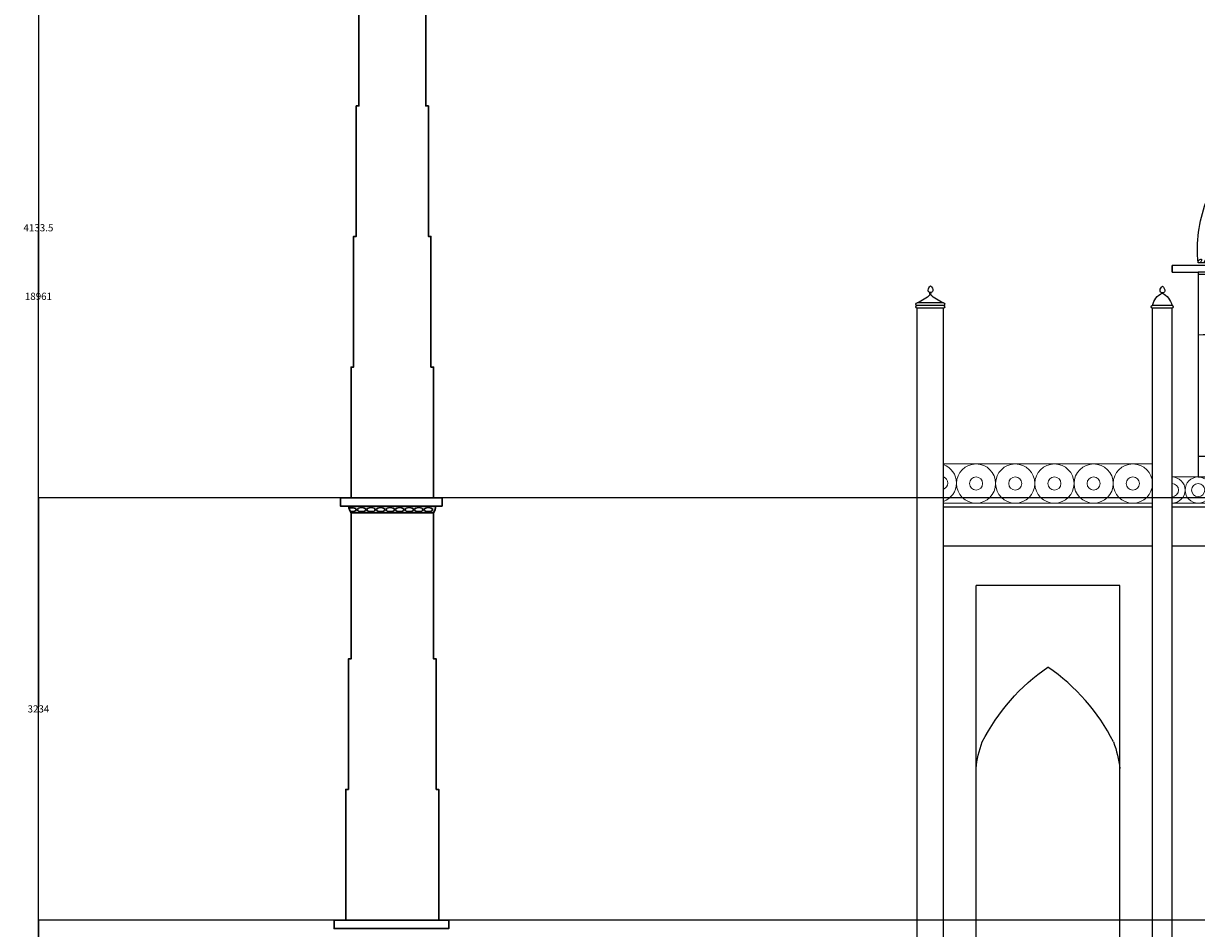
# Model space of a CAD drawing. Units: millimetres. Extents: x 8570 to 49085, y 3782 to 24863.
# Tile 2 of 15: x 8570 to 17549, y 10542 to 17471. Entities that reach past the tile are written whole.
import ezdxf

# ---------------------------------------------------------------- set-up
doc = ezdxf.new("R2010")
doc.units = ezdxf.units.MM
doc.header["$MEASUREMENT"] = 0
doc.header["$PDMODE"] = 3
for name, color, linetype, lineweight in [('A-ANNO-DIMS', 2, 'Continuous', 18), ('A-ELEV', 7, 'Continuous', 25), ('A-ELEV-ARCH', 7, 'Continuous', 25), ('A-ELEV-MNRT', 7, 'Continuous', 30), ('A-ELEV-ORNM', 7, 'Continuous', 13), ('A-ELEV-PIER', 7, 'Continuous', 25), ('A-ROOF-CHAT', 7, 'Continuous', 25)]:
    doc.layers.add(name, color=color, linetype=linetype, lineweight=lineweight)
doc.styles.get("Standard").update_dxf_attribs({"font": 'arial.ttf'})
doc.dimstyles.get("Standard").update_dxf_attribs({"dimtxt": 55, "dimasz": 0.18, "dimexe": 0.18, "dimexo": 0.0625, "dimgap": 0.09, "dimtad": 0, "dimtih": 1, "dimtoh": 1, "dimdec": 0, "dimzin": 0, "dimdsep": 46, "dimtxsty": 'Standard', "dimcen": 0.09, "dimadec": 0, "dimazin": 0, "dimtfac": 1, "dimtdec": 0, "dimtofl": 0, "dimtmove": 0, "dimatfit": 3, "dimfxl": 1, "dimtolj": 1, "dimtzin": 0, "dimarcsym": 0})

# ---------------------------------------------------------------- blocks, each defined once
blk = doc.blocks.new('MINARET-ELEV')
h = blk.add_hatch(color=256)
h.dxf.hatch_style = 1
edge = h.paths.add_edge_path()
edge.add_arc((788.1, 7879), 96, 347.52389, 357.31225, ccw=False)
edge.add_ellipse((859.2, 7847.7), major_axis=(31.8, 0), ratio=0.472441, start_angle=385.01443, end_angle=315.51296)
edge.add_arc((788.1, 7879), 96, 325.26025, 332.17741, ccw=False)
edge.add_line((867, 7824.3), (235, 7824.3))
edge.add_arc((313.9, 7879), 96, 182.68775, 214.73975, ccw=False)
edge.add_line((218, 7874.5), (884, 7874.5))
edge = h.paths.add_edge_path(flags=16)
edge.add_ellipse((494.2, 7847.7), major_axis=(31.8, 0), ratio=0.472441, start_angle=0, end_angle=360, ccw=False)
edge = h.paths.add_edge_path(flags=16)
edge.add_ellipse((567.2, 7847.7), major_axis=(31.8, 0), ratio=0.472441, start_angle=0, end_angle=360, ccw=False)
edge = h.paths.add_edge_path(flags=16)
edge.add_ellipse((421.2, 7847.7), major_axis=(31.8, 0), ratio=0.472441, start_angle=0, end_angle=360, ccw=False)
edge = h.paths.add_edge_path(flags=16)
edge.add_ellipse((640.2, 7847.7), major_axis=(31.8, 0), ratio=0.472441, start_angle=0, end_angle=360, ccw=False)
edge = h.paths.add_edge_path(flags=16)
edge.add_ellipse((348.2, 7847.7), major_axis=(31.8, 0), ratio=0.472441, start_angle=0, end_angle=360, ccw=False)
edge = h.paths.add_edge_path(flags=16)
edge.add_ellipse((713.2, 7847.7), major_axis=(31.8, 0), ratio=0.472441, start_angle=0, end_angle=360, ccw=False)
edge = h.paths.add_edge_path(flags=16)
edge.add_ellipse((275.2, 7847.7), major_axis=(31.8, 0), ratio=0.472441, start_angle=0, end_angle=360, ccw=False)
edge = h.paths.add_edge_path(flags=16)
edge.add_ellipse((786.2, 7847.7), major_axis=(31.8, 0), ratio=0.472441, start_angle=0, end_angle=360, ccw=False)
blk.add_line((867, 7824.3), (235, 7824.3))
blk.add_line((867, 7824.3), (235, 7824.3))
for points in [[(235, 7939), (235, 8939), (255, 8939), (255, 9939), (275, 9939), (275, 10939), (295, 10939), (295, 11939)], [(867, 7939), (867, 8939), (847, 8939), (847, 9939), (827, 9939), (827, 10939), (807, 10939), (807, 11939)], [(195, 4705), (195, 5705), (215, 5705), (215, 6705), (235, 6705), (235, 7824.3)], [(907, 4705), (907, 5705), (887, 5705), (887, 6705), (867, 6705), (867, 7824.3)]]:
    blk.add_lwpolyline(points)
for points in [[(948, 7939), (170.5, 7939), (170.5, 7874.5), (948, 7874.5)], [(997, 4705), (119.5, 4705), (119.5, 4640.5), (997, 4640.5)]]:
    blk.add_lwpolyline(points, close=True)
for centre, start, end in [((313.9, 7879), 182.68775, 214.73975), ((788.1, 7879), 325.26025, 357.31225)]:
    blk.add_arc(centre, 96, start, end)
at = {"extrusion": (0, 0, -1)}
for centre, start_param, end_param in [((275.2, 7847.7), -6.283185, 0), ((348.2, 7847.7), -6.283185, 0), ((421.2, 7847.7), -6.283185, 0), ((494.2, 7847.7), -6.283185, 0), ((567.2, 7847.7), -6.283185, 0), ((640.2, 7847.7), -6.283185, 0), ((713.2, 7847.7), -6.283185, 0), ((786.2, 7847.7), -6.283185, 0), ((859.2, 7847.7), -5.160703, -0.779193)]:
    blk.add_ellipse(centre, major_axis=(31.8, 0), ratio=0.472441, start_param=start_param, end_param=end_param, dxfattribs=at)
blk = doc.blocks.new('PAVILION-EDGE-PINNACLE')
for p, q in [((10, 8089.5), (160, 8089.5)), ((10, 0), (10, 8069.5)), ((10, 8069.5), (160, 8069.5)), ((160, 0), (160, 8069.5)), ((160, 0), (160, 6876.5)), ((10, 0), (10, 6246.5))]:
    blk.add_line(p, q)
blk.add_lwpolyline([(101.6, 8204.8, 0.216309), (82.9, 8236.3, 0.244698), (64, 8200, 0.244698)], format="xyb")
for centre, radius, start, end in [((153, 8055.1), 147, 117.52778, 166.47476), ((82.6, 8204.4), 19, 193.30654, 1.38797), ((17, 8055.1), 147, 13.52524, 62.47222), ((10, 8079.5), 10, 90, 270), ((160, 8079.5), 10, 270, 90)]:
    blk.add_arc(centre, radius, start, end)
blk = doc.blocks.new('WING-END-PINNACLE')
for p, q in [((10, 8109.5), (210, 8109.5)), ((10, 8089.5), (210, 8089.5)), ((10, 0), (10, 8069.5)), ((10, 8069.5), (210, 8069.5)), ((210, 0), (210, 8069.5))]:
    blk.add_line(p, q)
blk.add_lwpolyline([(127.1, 8207.4, 0.216309), (108.4, 8238.9, 0.244698), (89.5, 8202.5, 0.244698)], format="xyb")
blk.add_circle((110.5, 8181), 7.02)
for centre, radius, start, end in [((-119.7, 8420.4), 336.9, 292.6494, 312.99463), ((108.1, 8206.9), 19, 193.30654, 1.38797), ((340.2, 8421.1), 337.7, 227.0303, 247.32566), ((10, 8099.5), 10, 90, 270), ((10, 8079.5), 10, 90, 270), ((210, 8099.5), 10, 270, 90), ((210, 8079.5), 10, 270, 90)]:
    blk.add_arc(centre, radius, start, end)
blk = doc.blocks.new('ARCADE-RING-FRIEZE')
for p, q in [((0, 200), (2300, 200)), ((2300, 200), (2100, 200)), ((0, 0), (2300, 0))]:
    blk.add_line(p, q)
for centre, radius in [((100, 100), 100), ((300, 100), 100), ((500, 100), 100), ((700, 100), 100), ((900, 100), 100), ((1100, 100), 100), ((1300, 100), 100), ((1500, 100), 100), ((1700, 100), 100), ((1900, 100), 100), ((2100, 100), 100), ((100, 100), 50), ((300, 100), 50), ((500, 100), 50), ((700, 100), 50), ((900, 100), 50), ((1100, 100), 50), ((1300, 100), 50), ((1500, 100), 50), ((1700, 100), 50), ((1900, 100), 50), ((2100, 100), 50)]:
    blk.add_circle(centre, radius)
for radius in [100, 50]:
    blk.add_arc((2300, 100), radius, 90, 270)
blk = doc.blocks.new('WING-RING-FRIEZE')
for p, q in [((0, 300), (1600, 300)), ((0, 0), (1600, 0))]:
    blk.add_line(p, q)
for centre, radius in [((150, 150), 150), ((450, 150), 150), ((750, 150), 150), ((1050, 150), 150), ((1349.9, 150), 150), ((150, 150), 50), ((450, 150), 50), ((750, 150), 50), ((1050, 150), 50), ((1349.9, 150), 50)]:
    blk.add_circle(centre, radius)
for centre, radius in [((1649.9, 153.7), 150), ((1616.6, 153.7), 50)]:
    blk.add_arc(centre, radius, 109.41717, 250.58283)
blk = doc.blocks.new('CHHATRI-ELEV')
for p, q in [((1107.1, 3111.9), (1194.6, 3111.9)), ((819.3, 2507.3), (1150, 2958.1)), ((967.4, 2449.5), (1150, 2958.1)), ((1480.7, 2507.3), (1150, 2958.1)), ((1339.8, 2454.2), (1150, 2958.1)), ((200, 1639.5), (2100, 1639.5)), ((2300, 1569.5), (2300, 1619.5)), ((200, 1549.5), (2100, 1549.5)), ((610, 0), (610, 754)), ((800, 0), (800, 754)), ((1500, 0), (1500, 744.5)), ((1692, 0), (1692, 744.5)), ((610, 158.5), (200, 158.5)), ((800, 158.5), (1500, 158.5)), ((2100, 158.5), (1692, 158.5))]:
    blk.add_line(p, q)
for points in [[(1199.3, 3183.7, 0.216309), (1151.6, 3264, 0.244698), (1103.6, 3171.4, 0.244698)], [(1198.5, 3007.8, 0.216309), (1150.8, 3088.1, 0.244698), (1102.8, 2995.4, 0.244698)], [(259.6, 2102.5, -0.128405), (908.9, 2832.4, 0.03556), (1150, 2958.1)], [(2040.4, 2102.5, 0.128405), (1391.1, 2832.4, -0.03556), (1150, 2958.1)]]:
    blk.add_lwpolyline(points, format="xyb")
for points in [[(200, 1569.5), (0, 1569.5), (0, 1619.5), (2300, 1619.5), (2300, 1569.5), (2100, 1569.5)], [(2100, 0), (200, 0), (200, 1569.5), (2100, 1569.5), (2100, 0)]]:
    blk.add_lwpolyline(points)
for points in [[(225.8, 1639.5, 0.520567), (200.9, 1667.5, 0.520567)], [(273.9, 1639.5, 0.520567), (249, 1667.5, 0.520567)], [(321.9, 1639.5, 0.520567), (297.1, 1667.5, 0.520567)], [(370, 1639.5, 0.520567), (345.1, 1667.5, 0.520567)], [(418, 1639.5, 0.520567), (393.2, 1667.5, 0.520567)], [(466.1, 1639.5, 0.520567), (441.2, 1667.5, 0.520567)], [(514.2, 1639.5, 0.520567), (489.3, 1667.5, 0.520567)], [(562.2, 1639.5, 0.520567), (537.3, 1667.5, 0.520567)], [(610.3, 1639.5, 0.520567), (585.4, 1667.5, 0.520567)], [(658.3, 1639.5, 0.520567), (633.4, 1667.5, 0.520567)], [(706.4, 1639.5, 0.520567), (681.5, 1667.5, 0.520567)], [(754.4, 1639.5, 0.520567), (729.6, 1667.5, 0.520567)], [(802.5, 1639.5, 0.520567), (777.6, 1667.5, 0.520567)], [(850.5, 1639.5, 0.520567), (825.7, 1667.5, 0.520567)], [(898.6, 1639.5, 0.520567), (873.7, 1667.5, 0.520567)], [(946.7, 1639.5, 0.520567), (921.8, 1667.5, 0.520567)], [(994.7, 1639.5, 0.520567), (969.8, 1667.5, 0.520567)], [(1042.8, 1639.5, 0.520567), (1017.9, 1667.5, 0.520567)], [(1090.8, 1639.5, 0.520567), (1065.9, 1667.5, 0.520567)], [(1138.9, 1639.5, 0.520567), (1114, 1667.5, 0.520567)], [(1186.9, 1639.5, 0.520567), (1162.1, 1667.5, 0.520567)], [(1235, 1639.5, 0.520567), (1210.1, 1667.5, 0.520567)], [(1283, 1639.5, 0.520567), (1258.2, 1667.5, 0.520567)], [(1331.1, 1639.5, 0.520567), (1306.2, 1667.5, 0.520567)], [(1379.2, 1639.5, 0.520567), (1354.3, 1667.5, 0.520567)], [(1427.2, 1639.5, 0.520567), (1402.3, 1667.5, 0.520567)], [(1475.3, 1639.5, 0.520567), (1450.4, 1667.5, 0.520567)], [(1523.3, 1639.5, 0.520567), (1498.4, 1667.5, 0.520567)], [(1571.4, 1639.5, 0.520567), (1546.5, 1667.5, 0.520567)], [(1619.4, 1639.5, 0.520567), (1594.6, 1667.5, 0.520567)], [(1667.5, 1639.5, 0.520567), (1642.6, 1667.5, 0.520567)], [(1715.6, 1639.5, 0.520567), (1690.7, 1667.5, 0.520567)], [(1763.6, 1639.5, 0.520567), (1738.7, 1667.5, 0.520567)], [(1811.7, 1639.5, 0.520567), (1786.8, 1667.5, 0.520567)], [(1859.7, 1639.5, 0.520567), (1834.8, 1667.5, 0.520567)], [(1907.8, 1639.5, 0.520567), (1882.9, 1667.5, 0.520567)], [(1955.8, 1639.5, 0.520567), (1931, 1667.5, 0.520567)], [(2003.9, 1639.5, 0.520567), (1979, 1667.5, 0.520567)], [(2051.9, 1639.5, 0.520567), (2027.1, 1667.5, 0.520567)], [(2100, 1639.5, 0.520567), (2075.1, 1667.5, 0.520567)]]:
    blk.add_lwpolyline(points, format="xyb", close=True)
blk.add_circle((1150.8, 3100), 11.9)
for centre, radius, start, end in [((1150.8, 3182.5), 48.5, 193.30654, 1.38797), ((1150.8, 3079.7), 54.3, 36.37477, 143.62523), ((1150, 3006.6), 48.5, 193.30654, 1.38797), ((1145, 3123.8), 717.3, 225.15569, 315.39684), ((1145, 3123.8), 697.3, 225.15569, 315.39684), ((1217.2, 1743.8), 1022.5, 159.46554, 185.85431), ((1082.8, 1743.8), 1022.5, 354.14569, 20.53446), ((260.1, 742.6), 350.1, 358.13323, 99.88317), ((1149.9, 742.6), 350.1, 359.68831, 181.86677), ((2042.1, 742.6), 350.1, 80.47888, 180.31169)]:
    blk.add_arc(centre, radius, start, end)
blk = doc.blocks.new('WING-TALL-ARCH')
for p, q in [((0, 5946.5), (1100, 5946.5)), ((0, 0), (0, 5946.5)), ((1100, 0), (1100, 5946.5)), ((0, 3123.2), (1100, 3123.2))]:
    blk.add_line(p, q)
for points in [[(47.9, 4748, -0.124525), (550, 5321.3, -0.124525)], [(1052.1, 4748, 0.124525), (550, 5321.3, 0.124525)]]:
    blk.add_lwpolyline(points, format="xyb")
for centre, start, end in [((817.4, 4459.8), 159.46554, 174.14569), ((282.6, 4459.8), 5.85431, 20.53446)]:
    blk.add_arc(centre, 821.7, start, end)
blk = doc.blocks.new('*D44')
at = {"layer": 'A-ANNO-DIMS', "color": 0, "lineweight": -2, "transparency": 16777216}
for p, q in [((22399.7, 24863), (8684.3, 24863)), ((8684.5, 24862.8), (8684.5, 15410.4)), ((8684.5, 5901.7), (8684.5, 15354.1)), ((10843.9, 5901.5), (8684.3, 5901.5))]:
    blk.add_line(p, q, dxfattribs=at)
at = {"layer": 'A-ANNO-DIMS', "color": 0, "transparency": 16777216}
for points in [[(8684.5, 24862.8), (8684.5, 24862.8), (8684.5, 24863)], [(8684.5, 5901.7), (8684.5, 5901.7), (8684.5, 5901.5)]]:
    blk.add_solid(points, dxfattribs=at)
at = {"layer": 'Defpoints', "color": 0, "transparency": 16777216}
for p in [(8684.5, 24863), (22399.8, 24863), (10844, 5901.5)]:
    blk.add_point(p, dxfattribs=at)
at = {"layer": 'A-ANNO-DIMS', "color": 0, "transparency": 16777216, "insert": (8684.5, 15382.2), "char_height": 55, "attachment_point": 5}
blk.add_mtext('\\A1;18961', dxfattribs=at)
blk = doc.blocks.new('*D59')
at = {"layer": 'A-ANNO-DIMS', "color": 0, "lineweight": -2, "transparency": 16777216}
for p, q in [((32990.4, 10606.5), (8684.3, 10606.5)), ((8684.5, 10606.3), (8684.5, 8942.7)), ((8684.5, 7222.7), (8684.5, 8886.3)), ((32870.9, 7222.5), (8684.3, 7222.5))]:
    blk.add_line(p, q, dxfattribs=at)
at = {"layer": 'A-ANNO-DIMS', "color": 0, "transparency": 16777216}
for points in [[(8684.5, 10606.3), (8684.5, 10606.3), (8684.5, 10606.5)], [(8684.5, 7222.7), (8684.5, 7222.7), (8684.5, 7222.5)]]:
    blk.add_solid(points, dxfattribs=at)
at = {"layer": 'Defpoints', "color": 0, "transparency": 16777216}
for p in [(8684.5, 10606.5), (32990.5, 10606.5), (32871, 7222.5)]:
    blk.add_point(p, dxfattribs=at)
at = {"layer": 'A-ANNO-DIMS', "color": 0, "transparency": 16777216, "insert": (8684.5, 8914.5), "char_height": 55, "attachment_point": 5}
blk.add_mtext('\\A1;3384', dxfattribs=at)
blk = doc.blocks.new('*D60')
at = {"layer": 'A-ANNO-DIMS', "color": 0, "lineweight": -2, "transparency": 16777216}
for p, q in [((33041.4, 13840.5), (8684.3, 13840.5)), ((8684.5, 13840.3), (8684.5, 12251.7)), ((8684.5, 10606.7), (8684.5, 12195.3)), ((32990.4, 10606.5), (8684.3, 10606.5))]:
    blk.add_line(p, q, dxfattribs=at)
at = {"layer": 'A-ANNO-DIMS', "color": 0, "transparency": 16777216}
for points in [[(8684.5, 13840.3), (8684.5, 13840.3), (8684.5, 13840.5)], [(8684.5, 10606.7), (8684.5, 10606.7), (8684.5, 10606.5)]]:
    blk.add_solid(points, dxfattribs=at)
at = {"layer": 'Defpoints', "color": 0, "transparency": 16777216}
for p in [(8684.5, 13840.5), (33041.5, 13840.5), (32990.5, 10606.5)]:
    blk.add_point(p, dxfattribs=at)
at = {"layer": 'A-ANNO-DIMS', "color": 0, "transparency": 16777216, "insert": (8684.5, 12223.5), "char_height": 55, "attachment_point": 5}
blk.add_mtext('\\A1;3234', dxfattribs=at)
blk = doc.blocks.new('*D61')
at = {"layer": 'A-ANNO-DIMS', "color": 0, "lineweight": -2, "transparency": 16777216}
for p, q in [((33091.4, 17974), (8684.3, 17974)), ((8684.5, 17973.8), (8684.5, 15935.4)), ((8684.5, 13840.7), (8684.5, 15879.1)), ((33041.4, 13840.5), (8684.3, 13840.5))]:
    blk.add_line(p, q, dxfattribs=at)
at = {"layer": 'A-ANNO-DIMS', "color": 0, "transparency": 16777216}
for points in [[(8684.5, 17973.8), (8684.5, 17973.8), (8684.5, 17974)], [(8684.5, 13840.7), (8684.5, 13840.7), (8684.5, 13840.5)]]:
    blk.add_solid(points, dxfattribs=at)
at = {"layer": 'Defpoints', "color": 0, "transparency": 16777216}
for p in [(8684.5, 17974), (33091.5, 17974), (33041.5, 13840.5)]:
    blk.add_point(p, dxfattribs=at)
at = {"layer": 'A-ANNO-DIMS', "color": 0, "transparency": 16777216, "insert": (8684.5, 15907.2), "char_height": 55, "attachment_point": 5}
blk.add_mtext('\\A1;4133.5', dxfattribs=at)

msp = doc.modelspace()

# ---------------------------------------------------------------- linework, layer by layer
at = {"layer": 'A-ELEV'}
for p, q in [((17211, 13769), (15611, 13769)), ((19661, 13769), (17361, 13769)), ((17211, 13469), (15611, 13469)), ((19661, 13469), (17361, 13469))]:
    msp.add_line(p, q, dxfattribs=at)

# ---------------------------------------------------------------- block references
at = {"layer": 'A-ELEV-ARCH', "extrusion": (0, 0, -1), "zscale": -1}
msp.add_blockref('WING-TALL-ARCH', (-16961, 7222.5), dxfattribs=at)
at = {"layer": 'A-ELEV-MNRT', "extrusion": (0, 0, -1), "zscale": -1}
msp.add_blockref('MINARET-ELEV', (-11944, 5901.5), dxfattribs=at)
at = {"layer": 'A-ELEV-ORNM', "extrusion": (0, 0, -1), "zscale": -1}
for name, p in [('WING-RING-FRIEZE', (-17211, 13799)), ('ARCADE-RING-FRIEZE', (-19661, 13799))]:
    msp.add_blockref(name, p, dxfattribs=at)
at = {"layer": 'A-ELEV-PIER', "extrusion": (0, 0, -1), "zscale": -1}
for name, p in [('WING-END-PINNACLE', (-15621, 7222.5)), ('PAVILION-EDGE-PINNACLE', (-17371, 7222.5))]:
    msp.add_blockref(name, p, dxfattribs=at)
at = {"layer": 'A-ROOF-CHAT', "extrusion": (0, 0, -1), "zscale": -1}
msp.add_blockref('CHHATRI-ELEV', (-19661, 13999), dxfattribs=at)

# ---------------------------------------------------------------- dimensions: what is measured, and where the dimension line sits
at = {"layer": 'A-ANNO-DIMS'}
for base, p1, p2, override, picture, middle in [((8684.5, 24862.95), (10844, 5901.5), (22399.75, 24862.95), {"dimdec": 0, "dimlfac": 1, "dimrnd": 0, "dimzin": 0, "dimdsep": 46, "dimlunit": 2}, '*D44', (8684.5, 15382.23)), ((8684.5, 17974), (33041.5, 13840.5), (33091.5, 17974), {"dimdec": 1, "dimlfac": 1, "dimrnd": 0, "dimzin": 0, "dimdsep": 46, "dimlunit": 2}, '*D61', (8684.5, 15907.25)), ((8684.5, 13840.5), (32990.5, 10606.5), (33041.5, 13840.5), {"dimdec": 0, "dimlfac": 1, "dimrnd": 0, "dimzin": 0, "dimdsep": 46, "dimlunit": 2}, '*D60', (8684.5, 12223.5)), ((8684.5, 10606.5), (32871, 7222.5), (32990.5, 10606.5), {"dimdec": 0, "dimlfac": 1, "dimrnd": 0, "dimzin": 0, "dimdsep": 46, "dimlunit": 2}, '*D59', (8684.5, 8914.5))]:
    dim = msp.add_linear_dim(base=base, p1=p1, p2=p2, angle=90, dimstyle='Standard', override=override, dxfattribs=at)
    dim.commit()
    dim.dimension.update_dxf_attribs({"geometry": picture, "text_midpoint": middle})

doc.saveas('drawing.dxf')
